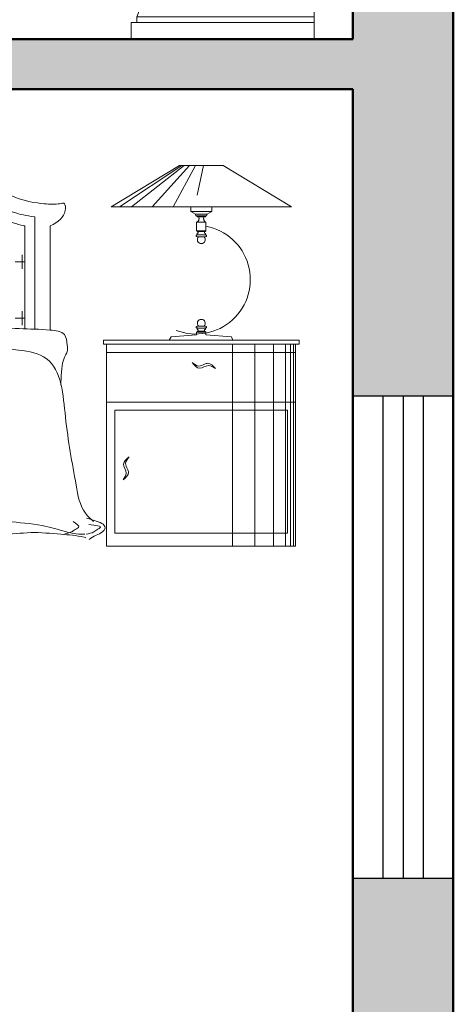
# Model space of a CAD drawing. Units: inches. Extents: x 1771 to 3025, y 319 to 889.
# Tile 29 of 35: x 2982 to 3025, y 521 to 619. Entities that reach past the tile are written whole.
import ezdxf

# ---------------------------------------------------------------- set-up
doc = ezdxf.new("R2010")
doc.units = ezdxf.units.IN
doc.header["$MEASUREMENT"] = 0
for name, color, linetype, lineweight in [('A-FLOR-FIXT', 8, 'Continuous', 18), ('A-FURN', 8, 'Continuous', 18), ('A-GLAZ', 40, 'Continuous', 25), ('A-WALL', 7, 'Continuous', 50), ('A-WALL-PATT', 254, 'Continuous', 13)]:
    doc.layers.add(name, color=color, linetype=linetype, lineweight=lineweight)

# ---------------------------------------------------------------- blocks, each defined once
blk = doc.blocks.new('A$C3908634B')
at = {"ltscale": 5}
for p, q in [((1200.2, 1046.3), (1218.1, 1046.3)), ((1176, 731), (1176, 731.7))]:
    blk.add_line(p, q, dxfattribs=at)
for p, q in [((1100.9, 962.2), (1134.6, 962.2)), ((1117.6, 945.1), (1117.6, 967.5)), ((1236.9, 962.2), (1271, 962.2)), ((1253.9, 945.1), (1253.9, 978.5)), ((184.3, 923.4), (19, 823.1)), ((237.5, 923.4), (184.3, 923.4)), ((190.2, 923.4), (237.5, 923.4)), ((231.9, 923.4), (247.3, 851.1)), ((284.7, 923.4), (237.5, 923.4)), ((237.5, 923.4), (290.6, 923.4)), ((251.7, 923.4), (305.7, 823.1)), ((266, 923.4), (356.4, 823.1)), ((278.7, 923.4), (406.8, 823.1)), ((284.7, 923.4), (436.3, 823.1)), ((290.6, 923.4), (456, 823.1)), ((1049.4, 876.9), (1049.4, 911)), ((1185.7, 876.9), (1185.7, 911)), ((1322.1, 876.9), (1322.1, 911)), ((2198.9, 923.4), (2033.5, 823.1)), ((2204.8, 923.4), (2053.3, 823.1)), ((2210.8, 923.4), (2082.7, 823.1)), ((2223.5, 923.4), (2133.1, 823.1)), ((2237.8, 923.4), (2183.8, 823.1)), ((2252, 923.4), (2198.9, 923.4)), ((2204.8, 923.4), (2252, 923.4)), ((2257.6, 923.4), (2242.2, 851.1)), ((2299.3, 923.4), (2252, 923.4)), ((2252, 923.4), (2305.2, 923.4)), ((2305.2, 923.4), (2470.5, 823.1)), ((1032.3, 894), (1066.4, 894)), ((1168.7, 894), (1202.8, 894)), ((1305.1, 894), (1339.1, 894)), ((940, 808.8), (940, 842.9)), ((1117.6, 808.8), (1117.6, 842.9)), ((1253.9, 808.8), (1253.9, 842.9)), ((1462.5, 808.8), (1462.5, 842.9)), ((237.5, 823.1), (19, 823.1)), ((212, 823.1), (212, 811.7)), ((237.5, 823.1), (456, 823.1)), ((263, 823.1), (263, 811.7)), ((741.7, 808.8), (741.7, 821.7)), ((746.2, 825.8), (758.8, 825.8)), ((922.9, 825.8), (957, 825.8)), ((1100.5, 825.8), (1134.6, 825.8)), ((1236.9, 825.8), (1271, 825.8)), ((1373.2, 825.8), (1479.5, 825.8)), ((1681.3, 808.8), (1681.3, 825.6)), ((2252, 823.1), (2033.5, 823.1)), ((2226.5, 823.1), (2226.5, 811.7)), ((2252, 823.1), (2470.5, 823.1)), ((2277.6, 823.1), (2277.6, 811.7)), ((212, 811.7), (223, 805.4)), ((212, 811.7), (237.5, 811.7)), ((223, 805.4), (224.6, 801.4)), ((223, 805.4), (237.5, 805.4)), ((250.4, 801.4), (224.6, 801.4)), ((226.9, 801.4), (228.3, 798.3)), ((228.3, 798.3), (237.5, 798.3)), ((228.3, 798.3), (231.3, 797.6)), ((231.1, 790.5), (230.2, 788)), ((231.5, 791.1), (231.1, 790.5)), ((231.3, 797.6), (232, 794.9)), ((231.6, 792.6), (231.5, 791.9)), ((231.5, 791.9), (231.5, 791.1)), ((231.9, 793.9), (231.6, 792.6)), ((232, 794.9), (231.9, 793.9)), ((263, 811.7), (237.5, 811.7)), ((252, 805.4), (237.5, 805.4)), ((246.7, 798.3), (237.5, 798.3)), ((243.7, 797.6), (243, 794.9)), ((243, 794.9), (243.1, 793.9)), ((243.1, 793.9), (243.4, 792.6)), ((243.4, 792.6), (243.4, 791.9)), ((243.4, 791.9), (243.4, 791.1)), ((243.4, 791.1), (243.9, 790.5)), ((246.7, 798.3), (243.7, 797.6)), ((243.9, 790.5), (244.8, 788)), ((248.1, 801.4), (246.7, 798.3)), ((252, 805.4), (250.4, 801.4)), ((263, 811.7), (252, 805.4)), ((621.3, 798.8), (621.3, 526)), ((1848.6, 798.8), (1848.6, 526.2)), ((2226.5, 811.7), (2237.6, 805.4)), ((2226.5, 811.7), (2252, 811.7)), ((2237.6, 805.4), (2239.1, 801.4)), ((2237.6, 805.4), (2252, 805.4)), ((2239.1, 801.4), (2264.9, 801.4)), ((2241.4, 801.4), (2242.8, 798.3)), ((2242.8, 798.3), (2245.8, 797.6)), ((2242.8, 798.3), (2252, 798.3)), ((2245.6, 790.5), (2244.7, 788)), ((2246.1, 791.1), (2245.6, 790.5)), ((2245.8, 797.6), (2246.5, 794.9)), ((2246.4, 793.9), (2246.1, 792.6)), ((2246.1, 792.6), (2246.1, 791.9)), ((2246.1, 791.9), (2246.1, 791.1)), ((2246.5, 794.9), (2246.4, 793.9)), ((2277.6, 811.7), (2252, 811.7)), ((2266.5, 805.4), (2252, 805.4)), ((2261.2, 798.3), (2252, 798.3)), ((2258.2, 797.6), (2257.6, 794.9)), ((2257.6, 794.9), (2257.6, 793.9)), ((2257.6, 793.9), (2257.9, 792.6)), ((2257.9, 792.6), (2258, 791.9)), ((2258, 791.9), (2258, 791.1)), ((2258, 791.1), (2258.4, 790.5)), ((2261.2, 798.3), (2258.2, 797.6)), ((2258.4, 790.5), (2259.4, 788)), ((2262.6, 801.4), (2261.2, 798.3)), ((2266.5, 805.4), (2264.9, 801.4)), ((2277.6, 811.7), (2266.5, 805.4)), ((227.8, 786.4), (226.2, 785.6)), ((226.2, 785.6), (226.2, 765)), ((226.2, 785.6), (248.8, 785.6)), ((226.2, 765), (227.6, 764.2)), ((226.2, 765), (237.5, 765)), ((227.6, 764.2), (228.5, 763.3)), ((230.2, 788), (227.8, 786.4)), ((248.8, 765), (237.5, 765)), ((244.8, 788), (247.2, 786.4)), ((247.4, 764.2), (246.5, 763.3)), ((247.2, 786.4), (248.8, 785.6)), ((248.8, 765), (247.4, 764.2)), ((248.8, 785.6), (248.8, 765)), ((645.8, 776.5), (645.8, 527)), ((673.5, 740.6), (673.5, 774.7)), ((809.9, 740.6), (809.9, 774.7)), ((1049.4, 740.6), (1049.4, 774.7)), ((1185.7, 740.6), (1185.7, 774.7)), ((1322.1, 740.6), (1322.1, 774.7)), ((1530.6, 751.3), (1530.6, 774.7)), ((1749.5, 740.6), (1749.5, 774.7)), ((1824, 776.5), (1824, 527.2)), ((2242.3, 786.4), (2240.7, 785.6)), ((2240.7, 785.6), (2240.7, 765)), ((2263.3, 785.6), (2240.7, 785.6)), ((2240.7, 765), (2242.1, 764.2)), ((2240.7, 765), (2252, 765)), ((2242.1, 764.2), (2243, 763.3)), ((2244.7, 788), (2242.3, 786.4)), ((2263.3, 765), (2252, 765)), ((2259.4, 788), (2261.7, 786.4)), ((2261.9, 764.2), (2261.1, 763.3)), ((2261.7, 786.4), (2263.3, 785.6)), ((2263.3, 765), (2261.9, 764.2)), ((2263.3, 785.6), (2263.3, 765)), ((224.8, 753.5), (224.7, 752.9)), ((224.7, 752.9), (224.8, 752.1)), ((225.3, 753.9), (224.8, 753.5)), ((224.8, 752.1), (225.2, 751.4)), ((225.2, 751.4), (225.6, 750.9)), ((225.7, 754.3), (225.3, 753.9)), ((225.6, 750.9), (228.1, 750.2)), ((226.3, 754.6), (225.7, 754.3)), ((227, 754.7), (226.3, 754.6)), ((227.9, 754.7), (227, 754.7)), ((227.4, 757.9), (227.1, 757.2)), ((227.1, 757.2), (227.3, 756.6)), ((227.3, 756.6), (227.8, 755.9)), ((227.7, 758.5), (227.4, 757.9)), ((228.6, 758.7), (227.7, 758.5)), ((227.8, 755.9), (228.9, 755.2)), ((228.9, 755.2), (227.9, 754.7)), ((228.1, 750.2), (229.9, 750)), ((228.5, 763.3), (229.4, 762.5)), ((228.5, 763.3), (237.5, 763.3)), ((229.4, 759.1), (228.6, 758.7)), ((228.9, 755.2), (237.5, 755.2)), ((229.4, 762.5), (230, 761.4)), ((229.8, 759.5), (229.4, 759.1)), ((230.1, 760.2), (229.8, 759.5)), ((229.9, 750), (232.4, 750.2)), ((230, 761.4), (230.1, 760.2)), ((232.4, 750.2), (237.5, 750.2)), ((246.5, 763.3), (237.5, 763.3)), ((246.1, 755.2), (237.5, 755.2)), ((242.6, 750.2), (237.5, 750.2)), ((245.1, 750), (242.6, 750.2)), ((245, 761.4), (244.9, 760.2)), ((244.9, 760.2), (245.2, 759.5)), ((245.6, 762.5), (245, 761.4)), ((246.9, 750.2), (245.1, 750)), ((245.2, 759.5), (245.6, 759.1)), ((246.5, 763.3), (245.6, 762.5)), ((245.6, 759.1), (246.4, 758.7)), ((247.2, 755.9), (246.1, 755.2)), ((246.1, 755.2), (247.1, 754.7)), ((246.4, 758.7), (247.3, 758.5)), ((249.4, 750.9), (246.9, 750.2)), ((247.1, 754.7), (248, 754.7)), ((247.7, 756.6), (247.2, 755.9)), ((247.3, 758.5), (247.6, 757.9)), ((247.6, 757.9), (247.9, 757.2)), ((247.9, 757.2), (247.7, 756.6)), ((248, 754.7), (248.7, 754.6)), ((248.7, 754.6), (249.3, 754.3)), ((249.3, 754.3), (249.7, 753.9)), ((249.8, 751.4), (249.4, 750.9)), ((249.7, 753.9), (250.2, 753.5)), ((250.2, 752.1), (249.8, 751.4)), ((250.2, 753.5), (250.3, 752.9)), ((250.3, 752.9), (250.2, 752.1)), ((656.5, 757.6), (690.6, 757.6)), ((792.9, 757.6), (827, 757.6)), ((1032.3, 757.6), (1066.4, 757.6)), ((1168.7, 757.6), (1202.8, 757.6)), ((1305.1, 757.6), (1339.1, 757.6)), ((1513.6, 757.6), (1547.7, 757.6)), ((1732.4, 757.6), (1766.5, 757.6)), ((2239.4, 753.5), (2239.2, 752.9)), ((2239.2, 752.9), (2239.3, 752.1)), ((2239.3, 752.1), (2239.7, 751.4)), ((2239.9, 753.9), (2239.4, 753.5)), ((2239.7, 751.4), (2240.2, 750.9)), ((2240.3, 754.3), (2239.9, 753.9)), ((2240.2, 750.9), (2242.6, 750.2)), ((2240.8, 754.6), (2240.3, 754.3)), ((2241.5, 754.7), (2240.8, 754.6)), ((2242.4, 754.7), (2241.5, 754.7)), ((2241.9, 757.9), (2241.7, 757.2)), ((2241.7, 757.2), (2241.8, 756.6)), ((2241.8, 756.6), (2242.3, 755.9)), ((2242.2, 758.5), (2241.9, 757.9)), ((2243.1, 758.7), (2242.2, 758.5)), ((2242.3, 755.9), (2243.4, 755.2)), ((2243.4, 755.2), (2242.4, 754.7)), ((2242.6, 750.2), (2244.4, 750)), ((2243, 763.3), (2243.9, 762.5)), ((2243, 763.3), (2252, 763.3)), ((2243.9, 759.1), (2243.1, 758.7)), ((2243.4, 755.2), (2252, 755.2)), ((2243.9, 762.5), (2244.6, 761.4)), ((2244.3, 759.5), (2243.9, 759.1)), ((2244.6, 760.2), (2244.3, 759.5)), ((2244.4, 750), (2246.9, 750.2)), ((2244.6, 761.4), (2244.6, 760.2)), ((2246.9, 750.2), (2252, 750.2)), ((2261.1, 763.3), (2252, 763.3)), ((2260.7, 755.2), (2252, 755.2)), ((2257.1, 750.2), (2252, 750.2)), ((2259.6, 750), (2257.1, 750.2)), ((2259.5, 761.4), (2259.4, 760.2)), ((2259.4, 760.2), (2259.7, 759.5)), ((2260.1, 762.5), (2259.5, 761.4)), ((2261.5, 750.2), (2259.6, 750)), ((2259.7, 759.5), (2260.1, 759.1)), ((2261.1, 763.3), (2260.1, 762.5)), ((2260.1, 759.1), (2260.9, 758.7)), ((2261.8, 755.9), (2260.7, 755.2)), ((2260.7, 755.2), (2261.6, 754.7)), ((2260.9, 758.7), (2261.8, 758.5)), ((2263.9, 750.9), (2261.5, 750.2)), ((2261.6, 754.7), (2262.5, 754.7)), ((2261.8, 758.5), (2262.2, 757.9)), ((2262.2, 756.6), (2261.8, 755.9)), ((2262.2, 757.9), (2262.4, 757.2)), ((2262.4, 757.2), (2262.2, 756.6)), ((2262.5, 754.7), (2263.2, 754.6)), ((2263.2, 754.6), (2263.8, 754.3)), ((2263.8, 754.3), (2264.2, 753.9)), ((2264.3, 751.4), (2263.9, 750.9)), ((2264.2, 753.9), (2264.7, 753.5)), ((2264.7, 752.1), (2264.3, 751.4)), ((2264.7, 753.5), (2264.8, 752.9)), ((2264.8, 752.9), (2264.7, 752.1)), ((741.7, 672.4), (741.7, 706.5)), ((940, 672.4), (940, 706.5)), ((1117.6, 672.4), (1117.6, 706.5)), ((1681.3, 672.4), (1681.3, 706.5)), ((1817.7, 672.4), (1817.7, 706.5)), ((724.7, 689.4), (758.8, 689.4)), ((922.9, 689.4), (957, 689.4)), ((1100.5, 689.4), (1134.6, 689.4)), ((1664.3, 689.4), (1698.3, 689.4)), ((1800.6, 689.4), (1824, 689.4)), ((656.5, 621.3), (690.6, 621.3)), ((673.5, 604.2), (673.5, 638.3)), ((792.9, 621.3), (823.2, 621.3)), ((809.9, 604.2), (809.9, 638.3)), ((1732.4, 621.3), (1766.5, 621.3)), ((1749.5, 604.2), (1749.5, 638.3)), ((724.7, 553.1), (758.8, 553.1)), ((741.7, 536), (741.7, 570.1)), ((1664.3, 553.1), (1698.3, 553.1)), ((1681.3, 536), (1681.3, 570.1)), ((1800.6, 553.1), (1824, 553.1)), ((1817.7, 536), (1817.7, 570.1)), ((224.7, 530.9), (224.8, 531.7)), ((224.8, 530.3), (224.7, 530.9)), ((224.8, 531.7), (225.2, 532.4)), ((225.3, 529.9), (224.8, 530.3)), ((225.2, 532.4), (225.6, 532.9)), ((225.7, 529.5), (225.3, 529.9)), ((225.6, 532.9), (228.1, 533.6)), ((226.3, 529.2), (225.7, 529.5)), ((227, 529.1), (226.3, 529.2)), ((227.9, 529.1), (227, 529.1)), ((227.1, 526.6), (227.3, 527.2)), ((227.4, 525.9), (227.1, 526.6)), ((227.3, 527.2), (227.8, 527.9)), ((227.7, 525.3), (227.4, 525.9)), ((228.6, 525.1), (227.7, 525.3)), ((227.8, 527.9), (228.9, 528.6)), ((228.9, 528.6), (227.9, 529.1)), ((228.1, 533.6), (229.9, 533.8)), ((228.9, 528.6), (237.5, 528.6)), ((230.3, 533.8), (237.5, 533.6)), ((242.6, 533.6), (237.5, 533.6)), ((246.1, 528.6), (237.5, 528.6)), ((245.1, 533.8), (242.6, 533.6)), ((246.9, 533.6), (245.1, 533.8)), ((246.1, 528.6), (247.1, 529.1)), ((247.2, 527.9), (246.1, 528.6)), ((246.4, 525.1), (247.3, 525.3)), ((249.4, 532.9), (246.9, 533.6)), ((247.1, 529.1), (248, 529.1)), ((247.7, 527.2), (247.2, 527.9)), ((247.3, 525.3), (247.6, 525.9)), ((247.6, 525.9), (247.9, 526.6)), ((247.9, 526.6), (247.7, 527.2)), ((248, 529.1), (248.7, 529.2)), ((248.7, 529.2), (249.3, 529.5)), ((249.3, 529.5), (249.7, 529.9)), ((249.8, 532.4), (249.4, 532.9)), ((249.7, 529.9), (250.2, 530.3)), ((250.2, 531.7), (249.8, 532.4)), ((250.3, 530.9), (250.2, 531.7)), ((250.2, 530.3), (250.3, 530.9)), ((2239.2, 530.9), (2239.3, 531.7)), ((2239.4, 530.3), (2239.2, 530.9)), ((2239.3, 531.7), (2239.7, 532.4)), ((2239.9, 529.9), (2239.4, 530.3)), ((2239.7, 532.4), (2240.2, 532.9)), ((2240.3, 529.5), (2239.9, 529.9)), ((2240.2, 532.9), (2242.6, 533.6)), ((2240.8, 529.2), (2240.3, 529.5)), ((2241.5, 529.1), (2240.8, 529.2)), ((2242.4, 529.1), (2241.5, 529.1)), ((2241.7, 526.6), (2241.8, 527.2)), ((2241.9, 525.9), (2241.7, 526.6)), ((2241.8, 527.2), (2242.3, 527.9)), ((2242.2, 525.3), (2241.9, 525.9)), ((2243.1, 525.1), (2242.2, 525.3)), ((2242.3, 527.9), (2243.4, 528.6)), ((2243.4, 528.6), (2242.4, 529.1)), ((2242.6, 533.6), (2244.4, 533.8)), ((2243.4, 528.6), (2252, 528.6)), ((2244.4, 533.8), (2246.9, 533.6)), ((2246.9, 533.6), (2252, 533.6)), ((2259.2, 533.8), (2252, 533.6)), ((2260.7, 528.6), (2252, 528.6)), ((2261.5, 533.6), (2259.6, 533.8)), ((2260.7, 528.6), (2261.6, 529.1)), ((2261.8, 527.9), (2260.7, 528.6)), ((2260.9, 525.1), (2261.8, 525.3)), ((2263.9, 532.9), (2261.5, 533.6)), ((2261.6, 529.1), (2262.5, 529.1)), ((2262.2, 527.2), (2261.8, 527.9)), ((2261.8, 525.3), (2262.2, 525.9)), ((2262.4, 526.6), (2262.2, 527.2)), ((2262.2, 525.9), (2262.4, 526.6)), ((2262.5, 529.1), (2263.2, 529.2)), ((2263.2, 529.2), (2263.8, 529.5)), ((2263.8, 529.5), (2264.2, 529.9)), ((2264.3, 532.4), (2263.9, 532.9)), ((2264.2, 529.9), (2264.7, 530.3)), ((2264.7, 531.7), (2264.3, 532.4)), ((2264.8, 530.9), (2264.7, 531.7)), ((2264.7, 530.3), (2264.8, 530.9)), ((164, 507.9), (161.1, 499.5)), ((164, 507.9), (226.2, 512.1)), ((226.2, 518.8), (227.6, 519.6)), ((226.2, 512.1), (226.2, 518.8)), ((226.2, 518.8), (237.5, 518.8)), ((227.6, 519.6), (228.5, 520.5)), ((228.5, 520.5), (229.4, 521.3)), ((229.4, 524.7), (228.6, 525.1)), ((229.8, 524.3), (229.4, 524.7)), ((229.4, 521.3), (230, 522.4)), ((229.4, 521.3), (237.5, 521.3)), ((230.1, 523.6), (229.8, 524.3)), ((230, 522.4), (230.1, 523.6)), ((245.6, 521.3), (237.5, 521.3)), ((248.8, 518.8), (237.5, 518.8)), ((244.9, 523.6), (245.2, 524.3)), ((245, 522.4), (244.9, 523.6)), ((245.6, 521.3), (245, 522.4)), ((245.2, 524.3), (245.6, 524.7)), ((245.6, 524.7), (246.4, 525.1)), ((246.5, 520.5), (245.6, 521.3)), ((247.4, 519.6), (246.5, 520.5)), ((248.8, 518.8), (247.4, 519.6)), ((248.8, 512.1), (248.8, 518.8)), ((311, 507.9), (248.8, 512.1)), ((311, 507.9), (315.3, 499.5)), ((2178.5, 507.9), (2174.2, 499.5)), ((2178.5, 507.9), (2240.7, 512.1)), ((2240.7, 518.8), (2242.1, 519.6)), ((2240.7, 512.1), (2240.7, 518.8)), ((2240.7, 518.8), (2252, 518.8)), ((2242.1, 519.6), (2243, 520.5)), ((2243, 520.5), (2243.9, 521.3)), ((2243.9, 524.7), (2243.1, 525.1)), ((2244.3, 524.3), (2243.9, 524.7)), ((2243.9, 521.3), (2244.6, 522.4)), ((2243.9, 521.3), (2252, 521.3)), ((2244.6, 523.6), (2244.3, 524.3)), ((2244.6, 522.4), (2244.6, 523.6)), ((2260.1, 521.3), (2252, 521.3)), ((2263.3, 518.8), (2252, 518.8)), ((2259.4, 523.6), (2259.7, 524.3)), ((2259.5, 522.4), (2259.4, 523.6)), ((2260.1, 521.3), (2259.5, 522.4)), ((2259.7, 524.3), (2260.1, 524.7)), ((2260.1, 524.7), (2260.9, 525.1)), ((2261.1, 520.5), (2260.1, 521.3)), ((2261.9, 519.6), (2261.1, 520.5)), ((2263.3, 518.8), (2261.9, 519.6)), ((2263.3, 512.1), (2263.3, 518.8)), ((2325.5, 507.9), (2263.3, 512.1)), ((2325.5, 507.9), (2328.4, 499.5)), ((475, 499.5), (0, 499.5)), ((0, 499.5), (0, 489.5)), ((475, 489.5), (0, 489.5)), ((8.7, 489.5), (8.7, 0)), ((14.1, 488.6), (14.1, 0)), ((21.3, 488.6), (21.3, 0)), ((33, 488.6), (33, 0)), ((62.7, 488.6), (62.7, 0)), ((107.6, 488.6), (107.6, 0)), ((161.1, 499.5), (237.5, 499.5)), ((161.6, 488.6), (161.6, 0)), ((315.3, 499.5), (237.5, 499.5)), ((467.1, 0), (467.1, 489.5)), ((475, 499.5), (475, 489.5)), ((2014.5, 499.5), (2489.5, 499.5)), ((2014.5, 499.5), (2014.5, 489.5)), ((2014.5, 489.5), (2489.5, 489.5)), ((2022.4, 0), (2022.4, 489.5)), ((2174.2, 499.5), (2252, 499.5)), ((2328.4, 499.5), (2252, 499.5)), ((2327.9, 488.6), (2327.9, 0)), ((2381.9, 488.6), (2381.9, 0)), ((2426.8, 488.6), (2426.8, 0)), ((2456.5, 488.6), (2456.5, 0)), ((2468.2, 488.6), (2468.2, 0)), ((2475.4, 488.6), (2475.4, 0)), ((2480.8, 489.5), (2480.8, 0)), ((2489.5, 499.5), (2489.5, 489.5)), ((467.1, 469.5), (8.7, 469.5)), ((2022.4, 469.5), (2480.8, 469.5)), ((467.1, 349.5), (8.7, 349.5)), ((2022.4, 349.5), (2480.8, 349.5)), ((28.7, 329.5), (28.7, 31.6)), ((447.1, 329.5), (28.7, 329.5)), ((447.1, 31.6), (447.1, 329.5)), ((2042.4, 329.5), (2460.8, 329.5)), ((2042.4, 31.6), (2042.4, 329.5)), ((2460.8, 329.5), (2460.8, 31.6)), ((467.1, 281.6), (467.1, 301.6)), ((2022.4, 281.6), (2022.4, 301.6)), ((28.7, 31.6), (447.1, 31.6)), ((2460.8, 31.6), (2042.4, 31.6)), ((8.7, 0), (467.1, 0)), ((2022.4, 0), (2480.8, 0))]:
    blk.add_line(p, q)
at = {"ltscale": 20}
for p, q in [((584.4, 776.7), (584.4, 523.7)), ((1885.4, 776.7), (1885.4, 524))]:
    blk.add_line(p, q, dxfattribs=at)
for centre, radius, start, end in [((1209.1, 956.2), 55.2, 80.5605, 99.4395), ((1209.1, 930.3), 55.2, 80.5605, 99.4395), ((250.5, 646.2), 131.8, 100.6234, 291.2), ((2239, 646.2), 131.8, 248.8, 79.3766), ((237.5, 743.5), 9.69, 137.7341, 270), ((237.5, 743.5), 9.69, 270, 42.2659), ((2252, 743.5), 9.69, 137.7341, 270), ((2252, 743.5), 9.69, 270, 42.2659), ((237.5, 540.3), 9.69, 90, 222.2659), ((237.5, 540.3), 9.69, 317.7341, 90), ((2252, 540.3), 9.69, 90, 222.2659), ((2252, 540.3), 9.69, 317.7341, 90)]:
    blk.add_arc(centre, radius, start, end)
for points in [[(584.4, 776.7), (563.9, 786.2), (546, 802.1), (547.3, 834.8), (564.5, 828.3), (620.6, 830.4), (706.4, 847.2), (752.1, 924.2), (778.1, 880.4), (846.1, 907.1), (1017.7, 1014.1), (1134.5, 1035.5), (1200.2, 1046.3)], [(1885.4, 776.7), (1905.9, 786.2), (1923.9, 802.1), (1922.5, 834.8), (1905.3, 828.3), (1849.2, 830.4), (1763.4, 847.2), (1717.7, 924.2), (1691.7, 880.4), (1541.2, 907.1), (1472.8, 1014.1), (1283.8, 1035.5), (1218.1, 1046.3)]]:
    blk.add_open_spline(points, degree=3, knots=[12.417853, 12.417853, 12.417853, 12.417853, 68.394536, 90.665986, 114.156853, 157.554067, 281.869614, 298.858744, 338.737111, 347.060176, 470.423438, 625.498764, 625.498764, 625.498764, 625.498764], dxfattribs=at)
for points, knots in [([(756.1, 861.8), (756.9, 861.3), (757.6, 860.9), (759.9, 859.6), (761.6, 858.7), (765.5, 856.8), (767.8, 855.8), (772.7, 854.1), (775.4, 853.3), (780.8, 852.2), (783.3, 851.8), (787.1, 851.6), (788.2, 851.5), (789.9, 851.5), (790.6, 851.5), (791.9, 851.5), (792.5, 851.5), (793.6, 851.6), (794.1, 851.6), (795.8, 851.8), (796.8, 851.9), (800.3, 852.3), (802.5, 852.8), (806.5, 853.8), (808.3, 854.3), (811.5, 855.4), (812.9, 855.9), (815.3, 856.9), (816.4, 857.4), (817.6, 857.9), (817.8, 858), (818.4, 858.2), (818.7, 858.4), (819.5, 858.7), (820, 859), (821.6, 859.7), (822.7, 860.2), (825.8, 861.7), (827.9, 862.8), (834, 866), (837.9, 868.3), (848.5, 874.9), (854.9, 879.4), (928.8, 888.8), (934.4, 893.5), (945, 903.2), (950, 908), (1000.9, 917.4), (1005.5, 922.1), (1014.4, 931), (1018.7, 935.3), (1027, 943.5), (1031.1, 947.3), (1036.9, 952.4), (1038.8, 954), (1042, 956.7), (1043.5, 957.9), (1045.8, 959.7), (1046.7, 960.3), (1048.5, 961.7), (1049.4, 962.3), (1052.1, 964.2), (1054, 965.5), (1059.7, 969.2), (1063.6, 971.5), (1074.8, 977.5), (1082.2, 980.9), (1098, 987.2), (1106.3, 990), (1123.7, 995.2), (1132.8, 997.5), (1151.5, 1001.8), (1161.1, 1003.8), (1180.5, 1007.4), (1190.2, 1009), (1200.1, 1010.7)], [328.6705, 328.6705, 328.6705, 328.6705, 329.609368, 329.609368, 331.487103, 331.487103, 333.620342, 333.620342, 335.753581, 335.753581, 337.507866, 337.507866, 338.182373, 338.182373, 338.607397, 338.607397, 338.959312, 338.959312, 339.311227, 339.311227, 340.015058, 340.015058, 341.722742, 341.722742, 343.430427, 343.430427, 345.138111, 345.138111, 346.845796, 346.845796, 347.37881, 347.37881, 347.911824, 347.911824, 348.977853, 348.977853, 351.109909, 351.109909, 355.374023, 355.374023, 363.902249, 363.902249, 379.258481, 379.258481, 394.614712, 394.614712, 409.970944, 409.970944, 425.327175, 425.327175, 440.683406, 440.683406, 456.039638, 456.039638, 463.285514, 463.285514, 469.01116, 469.01116, 472.593, 472.593, 476.17484, 476.17484, 483.338521, 483.338521, 497.665882, 497.665882, 522.309302, 522.309302, 546.952723, 546.952723, 571.596143, 571.596143, 596.239564, 596.239564, 619.876409, 619.876409, 619.876409, 619.876409]), ([(1713.7, 861.8), (1713, 861.3), (1712.2, 860.9), (1709.9, 859.6), (1708.2, 858.7), (1704.3, 856.8), (1702.1, 855.8), (1697.1, 854.1), (1694.4, 853.3), (1689.1, 852.2), (1686.5, 851.8), (1682.7, 851.6), (1681.7, 851.5), (1679.9, 851.5), (1679.2, 851.5), (1678, 851.5), (1677.4, 851.5), (1676.2, 851.6), (1675.7, 851.6), (1674.1, 851.8), (1673, 851.9), (1669.5, 852.3), (1667.3, 852.8), (1663.3, 853.8), (1661.5, 854.3), (1658.4, 855.4), (1657, 855.9), (1654.5, 856.9), (1653.4, 857.4), (1652.2, 857.9), (1652, 858), (1651.4, 858.2), (1651.2, 858.4), (1650.4, 858.7), (1649.8, 859), (1648.2, 859.7), (1647.1, 860.2), (1644, 861.7), (1641.9, 862.8), (1553.3, 866), (1549.4, 868.3), (1538.8, 874.9), (1532.4, 879.4), (1520.4, 888.8), (1514.8, 893.5), (1504.2, 903.2), (1499.2, 908), (1489.5, 917.4), (1484.9, 922.1), (1476.1, 931), (1471.8, 935.3), (1463.4, 943.5), (1459.4, 947.3), (1381.4, 952.4), (1379.5, 954), (1376.2, 956.7), (1374.8, 957.9), (1372.5, 959.7), (1371.6, 960.3), (1369.8, 961.7), (1368.9, 962.3), (1366.2, 964.2), (1364.3, 965.5), (1358.6, 969.2), (1354.6, 971.5), (1343.5, 977.5), (1336, 980.9), (1320.2, 987.2), (1311.9, 990), (1294.6, 995.2), (1285.5, 997.5), (1266.8, 1001.8), (1257.2, 1003.8), (1237.8, 1007.4), (1228.1, 1009), (1218.2, 1010.7)], [328.6705, 328.6705, 328.6705, 328.6705, 329.609368, 329.609368, 331.487103, 331.487103, 333.620342, 333.620342, 335.753581, 335.753581, 337.507866, 337.507866, 338.182373, 338.182373, 338.607397, 338.607397, 338.959312, 338.959312, 339.311227, 339.311227, 340.015058, 340.015058, 341.722742, 341.722742, 343.430427, 343.430427, 345.138111, 345.138111, 346.845796, 346.845796, 347.37881, 347.37881, 347.911824, 347.911824, 348.977853, 348.977853, 351.109909, 351.109909, 355.374023, 355.374023, 363.902249, 363.902249, 379.258481, 379.258481, 394.614712, 394.614712, 409.970943, 409.970943, 425.327175, 425.327175, 440.683406, 440.683406, 456.039637, 456.039637, 463.285514, 463.285514, 469.011154, 469.011154, 472.592992, 472.592992, 476.17483, 476.17483, 483.338506, 483.338506, 497.665857, 497.665857, 522.309275, 522.309275, 546.952693, 546.952693, 571.59611, 571.59611, 596.239528, 596.239528, 619.876409, 619.876409, 619.876409, 619.876409]), ([(756.1, 835.9), (756.9, 835.5), (757.6, 835), (759.9, 833.7), (761.6, 832.8), (765.5, 830.9), (767.8, 830), (772.7, 828.2), (775.4, 827.5), (780.8, 826.3), (783.3, 826), (787.1, 825.7), (788.2, 825.7), (789.9, 825.6), (790.6, 825.6), (791.9, 825.6), (792.5, 825.7), (793.6, 825.7), (794.1, 825.8), (795.8, 825.9), (796.8, 826), (800.3, 826.5), (802.5, 826.9), (806.5, 827.9), (808.3, 828.5), (811.5, 829.5), (812.9, 830.1), (815.3, 831), (816.4, 831.5), (817.6, 832), (817.8, 832.1), (818.4, 832.4), (818.7, 832.5), (819.5, 832.9), (820, 833.1), (821.6, 833.8), (822.7, 834.3), (825.8, 835.9), (827.9, 836.9), (834, 840.2), (837.9, 842.4), (848.5, 849), (854.9, 853.6), (928.8, 862.9), (934.4, 867.7), (945, 877.3), (950, 882.1), (1000.9, 891.6), (1005.5, 896.2), (1014.4, 905.2), (1018.7, 909.5), (1027, 917.6), (1031.1, 921.4), (1036.9, 926.6), (1038.8, 928.2), (1042, 930.9), (1043.5, 932), (1045.8, 933.8), (1046.7, 934.5), (1048.5, 935.8), (1049.4, 936.4), (1052.1, 938.4), (1054, 939.6), (1059.7, 943.3), (1063.6, 945.6), (1074.8, 951.6), (1082.2, 955), (1098, 961.3), (1106.3, 964.2), (1123.7, 969.3), (1132.8, 971.6), (1151.5, 975.9), (1161.1, 977.9), (1180.5, 981.5), (1190.2, 983.2), (1200.1, 984.8)], [328.6705, 328.6705, 328.6705, 328.6705, 329.609368, 329.609368, 331.487103, 331.487103, 333.620342, 333.620342, 335.753581, 335.753581, 337.507866, 337.507866, 338.182373, 338.182373, 338.607397, 338.607397, 338.959312, 338.959312, 339.311227, 339.311227, 340.015058, 340.015058, 341.722742, 341.722742, 343.430427, 343.430427, 345.138111, 345.138111, 346.845796, 346.845796, 347.37881, 347.37881, 347.911824, 347.911824, 348.977853, 348.977853, 351.109909, 351.109909, 355.374023, 355.374023, 363.902249, 363.902249, 379.258481, 379.258481, 394.614712, 394.614712, 409.970944, 409.970944, 425.327175, 425.327175, 440.683406, 440.683406, 456.039638, 456.039638, 463.285514, 463.285514, 469.01116, 469.01116, 472.593, 472.593, 476.17484, 476.17484, 483.338521, 483.338521, 497.665882, 497.665882, 522.309302, 522.309302, 546.952723, 546.952723, 571.596143, 571.596143, 596.239564, 596.239564, 619.876409, 619.876409, 619.876409, 619.876409]), ([(1713.7, 835.9), (1713, 835.5), (1712.2, 835), (1709.9, 833.7), (1708.2, 832.8), (1704.3, 830.9), (1702.1, 830), (1697.1, 828.2), (1694.4, 827.5), (1689.1, 826.3), (1686.5, 826), (1682.7, 825.7), (1681.7, 825.7), (1679.9, 825.6), (1679.2, 825.6), (1678, 825.6), (1677.4, 825.7), (1676.2, 825.7), (1675.7, 825.8), (1674.1, 825.9), (1673, 826), (1669.5, 826.5), (1667.3, 826.9), (1663.3, 827.9), (1661.5, 828.5), (1658.4, 829.5), (1657, 830.1), (1654.5, 831), (1653.4, 831.5), (1652.2, 832), (1652, 832.1), (1651.4, 832.4), (1651.2, 832.5), (1650.4, 832.9), (1649.8, 833.1), (1648.2, 833.8), (1647.1, 834.3), (1644, 835.9), (1641.9, 836.9), (1553.3, 840.2), (1549.4, 842.4), (1538.8, 849), (1532.4, 853.6), (1520.4, 862.9), (1514.8, 867.7), (1504.2, 877.3), (1499.2, 882.1), (1489.5, 891.6), (1484.9, 896.2), (1476.1, 905.2), (1471.8, 909.5), (1463.4, 917.6), (1459.4, 921.4), (1381.4, 926.6), (1379.5, 928.2), (1376.2, 930.9), (1374.8, 932), (1372.5, 933.8), (1371.6, 934.5), (1369.8, 935.8), (1368.9, 936.4), (1366.2, 938.4), (1364.3, 939.6), (1358.6, 943.3), (1354.6, 945.6), (1343.5, 951.6), (1336, 955), (1320.2, 961.3), (1311.9, 964.2), (1294.6, 969.3), (1285.5, 971.6), (1266.8, 975.9), (1257.2, 977.9), (1237.8, 981.5), (1228.1, 983.2), (1218.2, 984.8)], [328.6705, 328.6705, 328.6705, 328.6705, 329.609368, 329.609368, 331.487103, 331.487103, 333.620342, 333.620342, 335.753581, 335.753581, 337.507866, 337.507866, 338.182373, 338.182373, 338.607397, 338.607397, 338.959312, 338.959312, 339.311227, 339.311227, 340.015058, 340.015058, 341.722742, 341.722742, 343.430427, 343.430427, 345.138111, 345.138111, 346.845796, 346.845796, 347.37881, 347.37881, 347.911824, 347.911824, 348.977853, 348.977853, 351.109909, 351.109909, 355.374023, 355.374023, 363.902249, 363.902249, 379.258481, 379.258481, 394.614712, 394.614712, 409.970943, 409.970943, 425.327175, 425.327175, 440.683406, 440.683406, 456.039637, 456.039637, 463.285514, 463.285514, 469.011154, 469.011154, 472.592992, 472.592992, 476.17483, 476.17483, 483.338506, 483.338506, 497.665857, 497.665857, 522.309275, 522.309275, 546.952693, 546.952693, 571.59611, 571.59611, 596.239528, 596.239528, 619.876409, 619.876409, 619.876409, 619.876409]), ([(621.3, 798.8), (633.4, 799.9), (641.2, 801.3), (657.3, 805), (665.7, 807.2), (682.6, 812.8), (691.1, 816.1), (708.1, 824.2), (716.5, 828.9), (731.3, 839), (737.9, 844.1), (748.3, 853.5), (752.3, 857.5), (756.1, 861.8)], [179.330708, 179.330708, 179.330708, 179.330708, 196.086144, 196.086144, 213.445516, 213.445516, 230.804888, 230.804888, 248.16426, 248.16426, 262.451931, 262.451931, 271.832526, 271.832526, 271.832526, 271.832526]), ([(1848.6, 798.8), (1836.4, 799.9), (1828.6, 801.3), (1812.5, 805), (1804.1, 807.2), (1787.2, 812.8), (1778.7, 816.1), (1761.8, 824.2), (1753.4, 828.9), (1738.5, 839), (1731.9, 844.1), (1721.5, 853.5), (1717.5, 857.5), (1713.7, 861.8)], [179.400376, 179.400376, 179.400376, 179.400376, 196.086144, 196.086144, 213.445516, 213.445516, 230.804888, 230.804888, 248.16426, 248.16426, 262.451931, 262.451931, 271.832526, 271.832526, 271.832526, 271.832526]), ([(645.8, 776.5), (646.9, 776.7), (648, 777), (657.3, 779.1), (665.7, 781.3), (682.6, 786.9), (691.1, 790.3), (708.1, 798.3), (716.5, 803), (731.3, 813.1), (737.9, 818.2), (748.3, 827.7), (752.3, 831.7), (756.1, 835.9)], [193.740688, 193.740688, 193.740688, 193.740688, 196.086144, 196.086144, 213.445516, 213.445516, 230.804888, 230.804888, 248.16426, 248.16426, 262.451931, 262.451931, 271.832526, 271.832526, 271.832526, 271.832526]), ([(1824, 776.5), (1822.9, 776.7), (1821.8, 777), (1812.5, 779.1), (1804.1, 781.3), (1787.2, 786.9), (1778.7, 790.3), (1761.8, 798.3), (1753.4, 803), (1738.5, 813.1), (1731.9, 818.2), (1721.5, 827.7), (1717.5, 831.7), (1713.7, 835.9)], [193.740688, 193.740688, 193.740688, 193.740688, 196.086144, 196.086144, 213.445516, 213.445516, 230.804888, 230.804888, 248.16426, 248.16426, 262.451931, 262.451931, 271.832526, 271.832526, 271.832526, 271.832526]), ([(1512.2, 740.7), (1519.9, 740.7), (1533.1, 740.8), (1553.9, 735.5), (1652.4, 710.7), (1643.1, 675.3), (1648.8, 648.1), (1651.8, 634.5), (1651.9, 634)], [0, 0, 0, 0, 31.268494, 53.71641, 83.24833, 138.583941, 192.96698, 194.695488, 194.695488, 194.695488, 194.695488]), ([(1181.8, 730.2), (1176.9, 727.3), (1167.9, 723.5), (1152.3, 726.4), (1145.2, 713.6), (1142.1, 705.5), (1140.6, 701.2)], [16.588235, 16.588235, 16.588235, 16.588235, 39.368234, 56.465167, 72.647278, 91.317886, 91.317886, 91.317886, 91.317886]), ([(1167.2, 686.5), (1175.5, 684.3), (1192.8, 677.8), (1196.3, 659.6), (1197.1, 648.3)], [13.535772, 13.535772, 13.535772, 13.535772, 45.871957, 87.312392, 87.312392, 87.312392, 87.312392]), ([(849.2, 653.1), (844.3, 648.8), (832.7, 636.7), (919.4, 609.9), (841.8, 577.9), (927.1, 550.1), (918.1, 541), (854.7, 539.8)], [5.952535, 5.952535, 5.952535, 5.952535, 29.258845, 70.114919, 115.518645, 162.322231, 169.813565, 169.813565, 169.813565, 169.813565]), ([(259.6, 445.5), (254.3, 441.1), (244.8, 433.2), (231.9, 440.9), (217, 446), (209.2, 437.1), (203.4, 430.5)], [0, 0, 0, 0, 18.381528, 32.980054, 40.875646, 63.595153, 63.595153, 63.595153, 63.595153]), ([(259.6, 445.5), (254, 438.6), (242.8, 424.9), (221, 442.9), (208.9, 434.4), (203.4, 430.5)], [0, 0, 0, 0, 22.772447, 45.052082, 63.466582, 63.466582, 63.466582, 63.466582]), ([(2229.9, 445.5), (2235.6, 438.6), (2246.7, 424.9), (2268.5, 442.9), (2280.6, 434.4), (2286.1, 430.5)], [0, 0, 0, 0, 22.772447, 45.052082, 63.466582, 63.466582, 63.466582, 63.466582]), ([(2229.9, 445.5), (2235.2, 441.1), (2244.7, 433.2), (2257.6, 440.9), (2272.5, 446), (2280.3, 437.1), (2286.1, 430.5)], [0, 0, 0, 0, 18.381528, 32.980054, 40.875646, 63.595153, 63.595153, 63.595153, 63.595153]), ([(412.3, 216.6), (419.2, 211), (432.8, 199.9), (414.9, 178.1), (423.4, 166), (427.2, 160.5)], [0, 0, 0, 0, 22.772447, 45.052082, 63.466582, 63.466582, 63.466582, 63.466582]), ([(412.3, 216.6), (416.7, 211.4), (424.6, 201.9), (416.9, 189), (411.8, 174.1), (420.6, 166.3), (427.2, 160.5)], [0, 0, 0, 0, 18.381528, 32.980054, 40.875646, 63.595153, 63.595153, 63.595153, 63.595153]), ([(2077.2, 216.6), (2072.8, 211.4), (2064.9, 201.9), (2072.6, 189), (2077.8, 174.1), (2068.9, 166.3), (2062.3, 160.5)], [0, 0, 0, 0, 18.381528, 32.980054, 40.875646, 63.595153, 63.595153, 63.595153, 63.595153]), ([(2077.2, 216.6), (2070.3, 211), (2056.7, 199.9), (2074.6, 178.1), (2066.1, 166), (2062.3, 160.5)], [0, 0, 0, 0, 22.772447, 45.052082, 63.466582, 63.466582, 63.466582, 63.466582])]:
    blk.add_open_spline(points, degree=3, knots=knots)
at = {"ltscale": 5}
for points, knots in [([(1140.2, 671), (1140.5, 684.2), (1141, 702.6), (1139.6, 733.3), (1171.5, 732.8), (1207.8, 724.4), (1313, 731.7), (1377.9, 716.1), (1675.3, 776), (1653.6, 739.3), (1653.4, 708.6), (1656.7, 669.4), (1649.8, 624.8), (1652.8, 584.9), (1655.4, 559.2), (1656.8, 538.3)], [3.603347, 3.603347, 3.603347, 3.603347, 60.838375, 82.182907, 107.012175, 163.177093, 249.239778, 501.114283, 577.787612, 607.274607, 630.949286, 706.159707, 762.92633, 812.910096, 867.096105, 867.096105, 867.096105, 867.096105]), ([(853.1, 539.8), (853.8, 547.4), (919.3, 558.2), (845.3, 575.8), (836.7, 609.7), (818, 623.2), (814.4, 657.6), (840.5, 653), (943.6, 652.6), (1051.1, 671.7), (1127.7, 657.4), (1165, 689.4), (1205, 697), (1208.2, 671.1), (1198.6, 657.5), (1193.8, 634.4), (1197.9, 619.2), (1201.2, 597.1), (1215.4, 563.6), (1206.8, 549.2), (1203.5, 540.2)], [33.020195, 33.020195, 33.020195, 33.020195, 57.294753, 90.473933, 194.149416, 257.058105, 304.592565, 338.383824, 389.043604, 577.649845, 759.359611, 813.032269, 898.973184, 920.659088, 956.429806, 1000.911745, 1042.797508, 1121.842246, 1191.460876, 1213.109701, 1213.109701, 1213.109701, 1213.109701]), ([(533.2, 342.2), (554.6, 456.3), (543.3, 464.8), (546.8, 491.4), (549.9, 520.4), (602.8, 525.9), (675.3, 527.2), (929.2, 547.1), (1113.3, 536.9), (1259.7, 541.4)], [0, 0, 0, 0, 32.681627, 48.455722, 75.25348, 112.004017, 183.381957, 310.642358, 688.088714, 688.088714, 688.088714, 688.088714]), ([(1911, 390.4), (1911.9, 458.8), (1930, 464.8), (1926.5, 491.4), (1923.4, 520.4), (1870.5, 525.9), (1798, 527.2), (1556.5, 543.7), (1364.8, 538.4), (1259.7, 541.4)], [0, 0, 0, 0, 32.681627, 48.455722, 75.25348, 112.004017, 183.381957, 310.642358, 588.939547, 588.939547, 588.939547, 588.939547]), ([(482.8, 59.4), (489.8, 65.8), (514.7, 88.6), (517.4, 182.5), (520.5, 297.5), (551.9, 447.1), (697, 485.5), (926.3, 465.8), (1116.6, 468.9), (1210.9, 472.2)], [0, 0, 0, 0, 28.320233, 100.953775, 269.820348, 420.691469, 489.161544, 656.134073, 940.569207, 940.569207, 940.569207, 940.569207]), ([(1990.5, 59.4), (1983.5, 65.8), (1958.6, 88.6), (1942.6, 182.5), (1920.4, 297.5), (1912.1, 455.6), (1776.3, 485.5), (1526.4, 465.8), (1305.2, 468.9), (1210.9, 472.2)], [0, 0, 0, 0, 28.320233, 100.953775, 269.820348, 420.691469, 489.161544, 656.134073, 940.569207, 940.569207, 940.569207, 940.569207]), ([(682.9, 304.1), (695.4, 260.8), (719.1, 178.1), (730.8, 82.2), (753.9, 38.3), (757.8, 30.9)], [0, 0, 0, 0, 135.247847, 258.692787, 283.800228, 283.800228, 283.800228, 283.800228]), ([(1775.2, 304.1), (1762.7, 260.8), (1739, 178.1), (1727.3, 82.2), (1704.2, 38.3), (1700.3, 30.9)], [0, 0, 0, 0, 135.247847, 258.692787, 283.800228, 283.800228, 283.800228, 283.800228]), ([(682.9, 165.6), (688.3, 154.5), (703.5, 123.2), (710.2, 85), (723.1, 63.5), (724.6, 61.1)], [0, 0, 0, 0, 37.234018, 105.386078, 113.844905, 113.844905, 113.844905, 113.844905]), ([(1790.4, 165.6), (1785, 154.5), (1769.8, 123.2), (1763.1, 85), (1750.2, 63.5), (1748.7, 61.1)], [0, 0, 0, 0, 37.234018, 105.386078, 113.844905, 113.844905, 113.844905, 113.844905]), ([(482.8, 59.4), (474.7, 54.3), (464, 47.4), (477.3, 41.4), (486.1, 33.4), (496.5, 31.3), (502.9, 30)], [0, 0, 0, 0, 19.035414, 25.269998, 36.960672, 56.00812, 56.00812, 56.00812, 56.00812]), ([(504.2, 28.9), (509, 28.7), (522.4, 28.3), (553.7, 35.4), (605.7, 52.4), (665.1, 57), (705.3, 61.4), (721.5, 63.6), (724.2, 61.4), (724.6, 61.1)], [0, 0, 0, 0, 14.447875, 40.468341, 96.220884, 181.018327, 216.046098, 224.609189, 226.185962, 226.185962, 226.185962, 226.185962]), ([(1969.1, 28.9), (1964.3, 28.7), (1950.9, 28.3), (1919.6, 35.4), (1867.6, 52.4), (1808.2, 57), (1768, 61.4), (1751.8, 63.6), (1749.1, 61.4), (1748.7, 61.1)], [0, 0, 0, 0, 14.447875, 40.468341, 96.220884, 181.018327, 216.046098, 224.609189, 226.185962, 226.185962, 226.185962, 226.185962]), ([(1941.2, 59.4), (1949.3, 54.3), (1960, 47.4), (1946.7, 41.4), (1937.9, 33.4), (1927.5, 31.3), (1921, 30)], [0, 0, 0, 0, 19.035414, 25.269998, 36.960672, 56.00812, 56.00812, 56.00812, 56.00812]), ([(1979.3, 52.3), (1995.3, 50.6), (2014.9, 48.5), (1998.8, 40.1), (1989.9, 32.4), (1979.5, 30.2), (1973.1, 28.9)], [0, 0, 0, 0, 28.05485, 34.289435, 45.980108, 65.027556, 65.027556, 65.027556, 65.027556]), ([(1973.5, 67.9), (1979.4, 66.3), (1994.6, 62.3), (2025.5, 51), (2011.2, 31.6), (1995.7, 27.1), (1985.4, 20.1), (1979.9, 16.4)], [0, 0, 0, 0, 19.937155, 51.57724, 63.193909, 80.21631, 100.09061, 100.09061, 100.09061, 100.09061]), ([(704.5, 47.7), (683.7, 44.6), (656.6, 40.6), (582.3, 36), (604.8, 26.7), (618.5, 32.3), (643.5, 30.4), (675.7, 27.4), (715, 33.3), (758.1, 35.6), (793.8, 32.4), (824.3, 37.8), (918.5, 32.1), (952.2, 36.4), (1023, 23.8), (1044.1, 24.1), (1058.3, 21.3), (1065.7, 20.4)], [0, 0, 0, 0, 87.513803, 114.592793, 124.77702, 141.903576, 160.817021, 198.691115, 240.471478, 280.23486, 329.410006, 348.41762, 373.077233, 428.05708, 447.802257, 468.691939, 491.310217, 491.310217, 491.310217, 491.310217]), ([(1113.3, 28), (1122.2, 29.4), (1132.2, 31.9), (1141.4, 28.4), (1142.4, 28)], [516.212662, 516.212662, 516.212662, 516.212662, 542.681017, 546.007116, 546.007116, 546.007116, 546.007116]), ([(1200.5, 28), (1202, 28.4), (1222.7, 33.5), (1266.3, 36.8), (1334.2, 43.2), (1462.5, 35), (1502.7, 33.5), (1515.8, 41.2), (1520.7, 44.1)], [590.079786, 590.079786, 590.079786, 590.079786, 594.646549, 651.888327, 725.747367, 797.841373, 826.274406, 843.189267, 843.189267, 843.189267, 843.189267]), ([(1643.2, 35.6), (1652.1, 37), (1662.2, 39.5), (1671.4, 36), (1672.4, 35.6)], [516.212662, 516.212662, 516.212662, 516.212662, 542.681017, 546.007116, 546.007116, 546.007116, 546.007116]), ([(1972.3, 20.4), (1970.7, 20.8), (1950, 25.9), (1906.5, 29.2), (1838.6, 35.6), (1782.4, 27.4), (1742.2, 25.9), (1729.1, 33.6), (1724.3, 36.5)], [590.079786, 590.079786, 590.079786, 590.079786, 594.646549, 651.888327, 725.747367, 797.841373, 826.274406, 843.189267, 843.189267, 843.189267, 843.189267])]:
    blk.add_open_spline(points, degree=3, knots=knots, dxfattribs=at)
blk = doc.blocks.new('A$C062C426B')
for p, q in [((0.4867, 0.6739, -0.3429), (0.4867, 0.6365, -0.3429)), ((0.4992, 0.6739, -0.3429), (0.4867, 0.6739, -0.3429)), ((0.5616, 0.6739, -0.3429), (0.5491, 0.6739, -0.3429)), ((0.5616, 0.6365, -0.3429), (0.5616, 0.6739, -0.3429)), ((0.624, 0.649, -0.3429), (0.599, 0.6365, -0.3429)), ((0.624, 0.5491, -0.3429), (0.624, 0.649, -0.3429)), ((0.4867, 0.6365, -0.3429), (0.4992, 0.6365, -0.3429)), ((0.4992, 0.6365, -0.3429), (0.4992, 0.577, -0.3429)), ((0.5491, 0.6365, -0.3429), (0.5616, 0.6365, -0.3429)), ((0.5491, 0.577, -0.3429), (0.5491, 0.6365, -0.3429)), ((0.599, 0.624, -0.3429), (0.5491, 0.624, -0.3429)), ((0.599, 0.6365, -0.3429), (0.599, 0.5616, -0.3429)), ((0.5521, 0.5741, -0.3429), (0.599, 0.5741, -0.3429)), ((0.599, 0.5616, -0.3429), (0.624, 0.5491, -0.3429)), ((0.4867, 0.5117, -0.3429), (0.5017, 0.5192, -0.3429)), ((0.4867, 0.4992, -0.3429), (0.4867, 0.5117, -0.3429)), ((0.5616, 0.5117, -0.3429), (0.5466, 0.5192, -0.3429)), ((0.5616, 0.4992, -0.3429), (0.5616, 0.5117, -0.3429)), ((0.4867, 0.4992, -0.3429), (0.4992, 0.4992, -0.3429)), ((0.4992, 0.4118, -0.3429), (0.4992, 0.4992, -0.3429)), ((0.5491, 0.4118, -0.3429), (0.5491, 0.4992, -0.3429)), ((0.5491, 0.4992, -0.3429), (0.5616, 0.4992, -0.3429)), ((0.4243, 0.4243, -0.3429), (0.0125, 0.4243, -0.3429)), ((0.0125, 0.4243, -0.3429), (0.0125, 0.3994, -0.3429)), ((0.4243, 0.3994, -0.3429), (0.4243, 0.4243, -0.3429)), ((0.5616, 0.3994, -0.3429), (0, 0.3994, -0.3429)), ((0, 0.3994, -0.3429), (0, 0.337, -0.3429)), ((0.4992, 0.4118, -0.3429), (0.4867, 0.4118, -0.3429)), ((0.4867, 0.4118, -0.3429), (0.4867, 0.3994, -0.3429)), ((0.5616, 0.4118, -0.3429), (0.5491, 0.4118, -0.3429)), ((0.5616, 0.3994, -0.3429), (0.5616, 0.4118, -0.3429)), ((0.5741, 0.3869, -0.3429), (0.5741, 0.1761, -0.3429)), ((0, 0.337, -0.3429), (0.4493, 0.337, -0.3429)), ((0.567, 0.1504, -0.3429), (0.5438, 0.1117, -0.3429)), ((0.5366, 0.086, -0.3429), (0.5366, 0, -0.3429)), ((0.5366, 0.0499, -0.3429), (0.1373, 0.0499, -0.3429)), ((0.1373, 0.0499, -0.3429), (0.1373, 0.0374, -0.3429)), ((0.5366, 0.0374, -0.3429), (0.1248, 0.0374, -0.3429)), ((0.1248, 0.0374, -0.3429), (0.1248, 0, -0.3429))]:
    blk.add_line(p, q)
for radius in [0.0374, 0.0125]:
    blk.add_circle((0.5242, 0.5491, -0.3429), radius)
for centre, radius, start, end in [((0.5242, 0.6552, -0.3429), 0.0312, 36.8699, 143.1301), ((0.5616, 0.3869, -0.3429), 0.0125, 0, 90), ((0.5429, 0.181, -0.3429), 0.1819, 95.9061, 120.9638), ((0.2791, 0.4017, -0.3429), 0.2664, 194.0552, 310.7015), ((-0.0044, 0.1107, -0.3429), 0.1542, 336.7818, 25.8778), ((0.5242, 0.1761, -0.3429), 0.0499, 329.0362, 0), ((0.5866, 0.086, -0.3429), 0.0499, 149.0362, 180)]:
    blk.add_arc(centre, radius, start, end)
blk = doc.blocks.new('WIN-48')
for p, q in [((0, 0), (0, 10)), ((48, 0), (48, 10)), ((0, 7), (48, 7)), ((0, 5), (48, 5)), ((0, 3), (48, 3))]:
    blk.add_line(p, q)

msp = doc.modelspace()

# ---------------------------------------------------------------- hatches: boundary and pattern name
at = {"layer": 'A-WALL-PATT'}
h = msp.add_hatch(color=256, dxfattribs=at)
h.dxf.hatch_style = 1
h.paths.add_polyline_path([(2870.685, 879.484), (2892.728, 879.484), (2892.728, 889.484), (2842.685, 889.484), (2842.685, 879.484), (2865.685, 879.484), (2865.685, 831.484), (2870.685, 831.484)])
h.paths.add_polyline_path([(2983.637, 889.484), (2940.728, 889.484), (2940.728, 879.484), (2961.685, 879.484), (2961.685, 795.484), (2865.685, 795.484), (2865.685, 759.484), (2865.685, 665.484), (2870.685, 665.484), (2870.685, 712.85), (2870.685, 790.484), (2978.685, 790.484), (2978.685, 795.484), (2966.685, 795.484), (2966.685, 879.484), (2983.637, 879.484)])
h.paths.add_polyline_path([(3024.685, 889.484), (3001.637, 889.484), (3001.637, 879.484), (3014.685, 879.484), (3014.685, 790.484), (3014.685, 769.459), (3024.685, 769.459)])
h.paths.add_polyline_path([(3024.685, 721.459), (3014.685, 721.459), (3014.685, 670.484), (2906.685, 670.484), (2906.685, 665.484), (2925.685, 665.484), (2925.685, 653.484), (2930.685, 653.484), (2930.685, 665.484), (3014.685, 665.484), (3014.685, 650.024), (3024.685, 650.024)])
h.paths.add_polyline_path([(3024.685, 632.024), (3014.685, 632.024), (3014.685, 617.484), (2925.685, 617.484), (2906.685, 617.484), (2906.685, 612.484), (3014.685, 612.484), (3014.685, 581.957), (3024.685, 581.957)])
h.paths.add_polyline_path([(3024.685, 533.957), (3014.685, 533.957), (3014.685, 480.484), (2870.685, 480.484), (2870.685, 617.484), (2860.685, 617.484), (2860.685, 544.484), (2769.685, 544.484), (2769.685, 534.484), (2860.685, 534.484), (2860.685, 470.484), (3014.685, 470.484), (3014.685, 453.613), (3024.685, 453.613)])
h.paths.add_polyline_path([(3024.685, 405.613), (3014.685, 405.613), (3014.685, 394.484), (2860.685, 394.484), (2860.685, 384.484), (3024.685, 384.484)])
h.paths.add_polyline_path([(2733.685, 643.435), (2723.685, 643.435), (2723.685, 534.484), (2733.685, 534.484)])
h.paths.add_polyline_path([(2733.685, 754.484), (2829.685, 754.484), (2829.685, 759.484), (2733.685, 759.484), (2733.685, 843.439, -0.008336), (2732.382, 843.484), (2723.685, 843.484), (2723.685, 691.435), (2733.685, 691.435)])
h.paths.add_polyline_path([(2794.685, 889.484), (2723.685, 889.484), (2723.685, 879.484), (2794.685, 879.484)])

# ---------------------------------------------------------------- linework, layer by layer
at = {"layer": 'A-WALL'}
for p, q in [((3024.685, 384.484), (3024.685, 889.282)), ((3014.685, 617.484), (3014.685, 665.484)), ((3014.685, 617.484), (2925.685, 617.484)), ((3014.685, 612.484), (2906.685, 612.484)), ((3014.685, 480.484), (3014.685, 612.484))]:
    msp.add_line(p, q, dxfattribs=at)

# ---------------------------------------------------------------- block references
at = {"layer": 'A-FLOR-FIXT', "xscale": 44.17762020618112, "yscale": 44.17762020618112, "zscale": 44.17762020618112}
msp.add_blockref('A$C062C426B', (2987.118, 617.484, 15.147), dxfattribs=at)
at = {"layer": 'A-FURN', "xscale": 0.0410441893854556, "yscale": 0.0410441893854556, "zscale": 0.0410441893854556}
msp.add_blockref('A$C3908634B', (2907.17, 567.009), dxfattribs=at)
at = {"layer": 'A-GLAZ', "rotation": 270.0000000000027}
msp.add_blockref('WIN-48', (3014.685, 581.956), dxfattribs=at)

doc.saveas('drawing.dxf')
